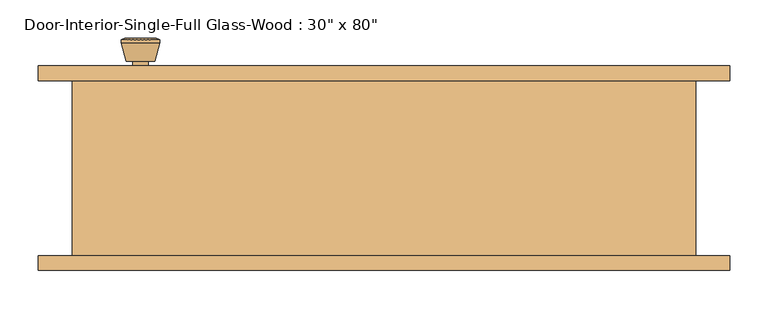
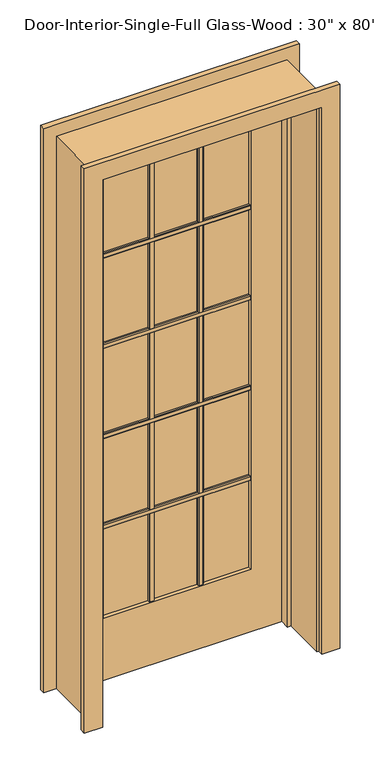
"""IFC4 building model written with IfcOpenShell, lengths in millimetres: door geometry."""

from ifc_helpers import new_model, si_unit, point, frame, frame_2d, origin, place, context, project, spatial, polyline, circle_curve, trimmed, segment, composite_curve, outline, extrude, faceted_brep, source, transform, mapped, element, save
from ifc_brep_helpers import plane_surface, cylinder_surface, revolved_surface, advanced_brep


def door_efd3daa1(model_context):
    return source(origin(), model_context, "Body", "SolidModel", [
        extrude(outline(polyline([(97.155, 1586.23), (103.505, 1586.23), (106.68, 1583.055), (106.68, 1570.355), (103.505, 1567.18), (97.155, 1567.18), (97.155, 1586.23)])), frame((-260.35, 0.0, 0.0), z_axis=(1.0, 0.0, 0.0), x_axis=(0.0, 1.0, 0.0)), (0.0, 0.0, 1.0), 520.7),
        extrude(outline(polyline([(97.155, 1249.9975), (103.505, 1249.9975), (106.68, 1246.8225), (106.68, 1234.1225), (103.505, 1230.9475), (97.155, 1230.9475), (97.155, 1249.9975)])), frame((-260.35, 0.0, 0.0), z_axis=(1.0, 0.0, 0.0), x_axis=(0.0, 1.0, 0.0)), (0.0, 0.0, 1.0), 520.7),
        extrude(outline(polyline([(97.155, 913.765), (103.505, 913.765), (106.68, 910.59), (106.68, 897.89), (103.505, 894.715), (97.155, 894.715), (97.155, 913.765)])), frame((-260.35, 0.0, 0.0), z_axis=(1.0, 0.0, 0.0), x_axis=(0.0, 1.0, 0.0)), (0.0, 0.0, 1.0), 520.7),
        extrude(outline(polyline([(97.155, 577.5325), (103.505, 577.5325), (106.68, 574.3575), (106.68, 561.6575), (103.505, 558.4825), (97.155, 558.4825), (97.155, 577.5325)])), frame((-260.35, 0.0, 0.0), z_axis=(1.0, 0.0, 0.0), x_axis=(0.0, 1.0, 0.0)), (0.0, 0.0, 1.0), 520.7),
        extrude(outline(polyline([(77.2583333, 97.155), (77.2583333, 103.505), (80.4333333, 106.68), (93.1333333, 106.68), (96.3083333, 103.505), (96.3083333, 97.155), (77.2583333, 97.155)])), frame((0.0, 0.0, 231.775), z_axis=(0.0, 0.0, 1.0), x_axis=(1.0, 0.0, 0.0)), (0.0, 0.0, 1.0), 1681.1625),
        extrude(outline(polyline([(-96.3083333, 97.155), (-96.3083333, 103.505), (-93.1333333, 106.68), (-80.4333333, 106.68), (-77.2583333, 103.505), (-77.2583333, 97.155), (-96.3083333, 97.155)])), frame((0.0, 0.0, 231.775), z_axis=(0.0, 0.0, 1.0), x_axis=(1.0, 0.0, 0.0)), (0.0, 0.0, 1.0), 1681.1625),
        extrude(outline(polyline([(90.17, 1586.23), (90.17, 1567.18), (83.82, 1567.18), (80.645, 1570.355), (80.645, 1583.055), (83.82, 1586.23), (90.17, 1586.23)])), frame((-260.35, 0.0, 0.0), z_axis=(1.0, 0.0, 0.0), x_axis=(0.0, 1.0, 0.0)), (0.0, 0.0, 1.0), 520.7),
        extrude(outline(polyline([(90.17, 1249.9975), (90.17, 1230.9475), (83.82, 1230.9475), (80.645, 1234.1225), (80.645, 1246.8225), (83.82, 1249.9975), (90.17, 1249.9975)])), frame((-260.35, 0.0, 0.0), z_axis=(1.0, 0.0, 0.0), x_axis=(0.0, 1.0, 0.0)), (0.0, 0.0, 1.0), 520.7),
        extrude(outline(polyline([(90.17, 913.765), (90.17, 894.715), (83.82, 894.715), (80.645, 897.89), (80.645, 910.59), (83.82, 913.765), (90.17, 913.765)])), frame((-260.35, 0.0, 0.0), z_axis=(1.0, 0.0, 0.0), x_axis=(0.0, 1.0, 0.0)), (0.0, 0.0, 1.0), 520.7),
        extrude(outline(polyline([(90.17, 577.5325), (90.17, 558.4825), (83.82, 558.4825), (80.645, 561.6575), (80.645, 574.3575), (83.82, 577.5325), (90.17, 577.5325)])), frame((-260.35, 0.0, 0.0), z_axis=(1.0, 0.0, 0.0), x_axis=(0.0, 1.0, 0.0)), (0.0, 0.0, 1.0), 520.7),
        extrude(outline(polyline([(77.2583333, 90.17), (96.3083333, 90.17), (96.3083333, 83.82), (93.1333333, 80.645), (80.4333333, 80.645), (77.2583333, 83.82), (77.2583333, 90.17)])), frame((0.0, 0.0, 231.775), z_axis=(0.0, 0.0, 1.0), x_axis=(1.0, 0.0, 0.0)), (0.0, 0.0, 1.0), 1681.1625),
        extrude(outline(polyline([(-96.3083333, 90.17), (-77.2583333, 90.17), (-77.2583333, 83.82), (-80.4333333, 80.645), (-93.1333333, 80.645), (-96.3083333, 83.82), (-96.3083333, 90.17)])), frame((0.0, 0.0, 231.775), z_axis=(0.0, 0.0, 1.0), x_axis=(1.0, 0.0, 0.0)), (0.0, 0.0, 1.0), 1681.1625),
        advanced_brep(
        [(-317.5, 70.2, 914.4), (-307.5, 70.2, 914.4), (-327.5, 70.2, 914.4), (-297.0241324, 21.2, 914.4), (-317.5, 21.2, 914.4), (-337.9758676, 21.2, 914.4), (-292.5, 23.0278681, 914.4), (-342.5, 23.0278681, 914.4), (-292.5, 26.4915463, 914.4), (-342.5, 26.4915463, 914.4), (-298.863764, 51.2, 914.4), (-336.136236, 51.2, 914.4), (-307.5, 51.2, 914.4), (-327.5, 51.2, 914.4)],
        [
            (0, 1),
            (1, 2, circle_curve(frame((-317.5, 70.2, 914.4), z_axis=(0.0, 1.0, 0.0), x_axis=(-1.0, 0.0, 0.0)), 10.0)),
            (2, 0),
            (2, 1, circle_curve(frame((-317.5, 70.2, 914.4), z_axis=(0.0, 1.0, 0.0), x_axis=(-1.0, 0.0, 0.0)), 10.0)),
            (3, 4),
            (4, 5),
            (5, 3, circle_curve(frame((-317.5, 21.2, 914.4), z_axis=(0.0, -1.0, 0.0), x_axis=(-1.0, 0.0, 0.0)), 20.4758676)),
            (3, 5, circle_curve(frame((-317.5, 21.2, 914.4), z_axis=(0.0, -1.0, 0.0), x_axis=(-1.0, 0.0, 0.0)), 20.4758676)),
            (6, 3),
            (5, 7),
            (7, 6, circle_curve(frame((-317.5, 23.0278681, 914.4), z_axis=(0.0, -1.0, 0.0), x_axis=(-1.0, 0.0, 0.0)), 25.0)),
            (6, 7, circle_curve(frame((-317.5, 23.0278681, 914.4), z_axis=(0.0, -1.0, 0.0), x_axis=(-1.0, 0.0, 0.0)), 25.0)),
            (8, 6),
            (7, 9),
            (9, 8, circle_curve(frame((-317.5, 26.4915463, 914.4), z_axis=(0.0, -1.0, 0.0), x_axis=(-1.0, 0.0, 0.0)), 25.0)),
            (8, 9, circle_curve(frame((-317.5, 26.4915463, 914.4), z_axis=(0.0, -1.0, 0.0), x_axis=(-1.0, 0.0, 0.0)), 25.0)),
            (10, 8),
            (9, 11),
            (11, 10, circle_curve(frame((-317.5, 51.2, 914.4), z_axis=(0.0, -1.0, 0.0), x_axis=(-1.0, 0.0, 0.0)), 18.636236)),
            (10, 11, circle_curve(frame((-317.5, 51.2, 914.4), z_axis=(0.0, -1.0, 0.0), x_axis=(-1.0, 0.0, 0.0)), 18.636236)),
            (12, 10),
            (11, 13),
            (13, 12, circle_curve(frame((-317.5, 51.2, 914.4), z_axis=(0.0, -1.0, 0.0), x_axis=(-1.0, 0.0, 0.0)), 10.0)),
            (12, 13, circle_curve(frame((-317.5, 51.2, 914.4), z_axis=(0.0, -1.0, 0.0), x_axis=(-1.0, 0.0, 0.0)), 10.0)),
            (1, 12),
            (13, 2),
        ],
        [
            plane_surface(frame((-317.5, 70.2, 914.4), z_axis=(0.0, 1.0, 0.0), x_axis=(-1.0, 0.0, 0.0))),
            plane_surface(frame((-317.5, 21.2, 914.4), z_axis=(0.0, -1.0, 0.0), x_axis=(-1.0, 0.0, 0.0))),
            revolved_surface(polyline([(-337.9758676, 21.2, 914.4), (-342.5, 23.0278681, 914.4)]), (-317.5, 70.2, 914.4), (0.0, 1.0, 0.0)),
            cylinder_surface(frame((-317.5, 70.2, 914.4), z_axis=(0.0, 1.0, 0.0), x_axis=(-1.0, 0.0, 0.0)), 25.0),
            revolved_surface(polyline([(-342.5, 26.4915463, 914.4), (-336.136236, 51.2, 914.4)]), (-317.5, 70.2, 914.4), (0.0, 1.0, 0.0)),
            plane_surface(frame((-317.5, 51.2, 914.4), z_axis=(0.0, 1.0, 0.0), x_axis=(-1.0, 0.0, 0.0))),
            cylinder_surface(frame((-317.5, 70.2, 914.4), z_axis=(0.0, 1.0, 0.0), x_axis=(-1.0, 0.0, 0.0)), 10.0),
        ],
        [
            (0, [[1, 2, 3]]),
            (0, [[-3, 4, -1]]),
            (1, [[5, 6, 7]]),
            (1, [[-6, -5, 8]]),
            (2, [[9, -7, 10, 11]]),
            (2, [[-10, -8, -9, 12]]),
            (3, [[13, -11, 14, 15]]),
            (3, [[-14, -12, -13, 16]]),
            (4, [[17, -15, 18, 19]]),
            (4, [[-18, -16, -17, 20]]),
            (5, [[21, -19, 22, 23]]),
            (5, [[-22, -20, -21, 24]]),
            (6, [[25, -23, 26, -2]]),
            (6, [[-26, -24, -25, -4]]),
        ],
    ),
        extrude(outline(composite_curve([segment(trimmed(circle_curve(frame_2d((914.4, -317.5)), 30.0), [point((914.4, -347.5))], [point((914.4, -287.5))], False, "CARTESIAN"), True, "CONTINUOUS"), segment(trimmed(circle_curve(frame_2d((914.4, -317.5)), 30.0), [point((914.4, -287.5))], [point((914.4, -347.5))], False, "CARTESIAN"), True, "CONTINUOUS")], self_intersect=False)), frame((0.0, 70.2, 0.0), z_axis=(0.0, 1.0, 0.0), x_axis=(0.0, 0.0, 1.0)), (0.0, 0.0, 1.0), 6.0),
        advanced_brep(
        [(-317.5, 117.125, 914.4), (-327.5, 117.125, 914.4), (-307.5, 117.125, 914.4), (-297.0241324, 166.125, 914.4), (-337.9758676, 166.125, 914.4), (-317.5, 166.125, 914.4), (-292.5, 164.2971319, 914.4), (-342.5, 164.2971319, 914.4), (-292.5, 160.8334537, 914.4), (-342.5, 160.8334537, 914.4), (-298.863764, 136.125, 914.4), (-336.136236, 136.125, 914.4), (-307.5, 136.125, 914.4), (-327.5, 136.125, 914.4)],
        [
            (0, 1),
            (1, 2, circle_curve(frame((-317.5, 117.125, 914.4), z_axis=(0.0, -1.0, 0.0), x_axis=(-1.0, 0.0, 0.0)), 10.0)),
            (2, 0),
            (2, 1, circle_curve(frame((-317.5, 117.125, 914.4), z_axis=(0.0, -1.0, 0.0), x_axis=(-1.0, 0.0, 0.0)), 10.0)),
            (3, 4, circle_curve(frame((-317.5, 166.125, 914.4), z_axis=(0.0, 1.0, 0.0), x_axis=(-1.0, 0.0, 0.0)), 20.4758676)),
            (4, 5),
            (5, 3),
            (4, 3, circle_curve(frame((-317.5, 166.125, 914.4), z_axis=(0.0, 1.0, 0.0), x_axis=(-1.0, 0.0, 0.0)), 20.4758676)),
            (6, 7, circle_curve(frame((-317.5, 164.2971319, 914.4), z_axis=(0.0, 1.0, 0.0), x_axis=(-1.0, 0.0, 0.0)), 25.0)),
            (7, 4),
            (3, 6),
            (7, 6, circle_curve(frame((-317.5, 164.2971319, 914.4), z_axis=(0.0, 1.0, 0.0), x_axis=(-1.0, 0.0, 0.0)), 25.0)),
            (8, 9, circle_curve(frame((-317.5, 160.8334537, 914.4), z_axis=(0.0, 1.0, 0.0), x_axis=(-1.0, 0.0, 0.0)), 25.0)),
            (9, 7),
            (6, 8),
            (9, 8, circle_curve(frame((-317.5, 160.8334537, 914.4), z_axis=(0.0, 1.0, 0.0), x_axis=(-1.0, 0.0, 0.0)), 25.0)),
            (10, 11, circle_curve(frame((-317.5, 136.125, 914.4), z_axis=(0.0, 1.0, 0.0), x_axis=(-1.0, 0.0, 0.0)), 18.636236)),
            (11, 9),
            (8, 10),
            (11, 10, circle_curve(frame((-317.5, 136.125, 914.4), z_axis=(0.0, 1.0, 0.0), x_axis=(-1.0, 0.0, 0.0)), 18.636236)),
            (12, 13, circle_curve(frame((-317.5, 136.125, 914.4), z_axis=(0.0, 1.0, 0.0), x_axis=(-1.0, 0.0, 0.0)), 10.0)),
            (13, 11),
            (10, 12),
            (13, 12, circle_curve(frame((-317.5, 136.125, 914.4), z_axis=(0.0, 1.0, 0.0), x_axis=(-1.0, 0.0, 0.0)), 10.0)),
            (1, 13),
            (12, 2),
        ],
        [
            plane_surface(frame((-317.5, 117.125, 914.4), z_axis=(0.0, -1.0, 0.0), x_axis=(-1.0, 0.0, 0.0))),
            plane_surface(frame((-317.5, 166.125, 914.4), z_axis=(0.0, 1.0, 0.0), x_axis=(-1.0, 0.0, 0.0))),
            revolved_surface(polyline([(-337.9758676, 166.125, 914.4), (-342.5, 164.2971319, 914.4)]), (-317.5, 117.125, 914.4), (0.0, -1.0, 0.0)),
            cylinder_surface(frame((-317.5, 117.125, 914.4), z_axis=(0.0, -1.0, 0.0), x_axis=(-1.0, 0.0, 0.0)), 25.0),
            revolved_surface(polyline([(-342.5, 160.8334537, 914.4), (-336.136236, 136.125, 914.4)]), (-317.5, 117.125, 914.4), (0.0, -1.0, 0.0)),
            plane_surface(frame((-317.5, 136.125, 914.4), z_axis=(0.0, -1.0, 0.0), x_axis=(-1.0, 0.0, 0.0))),
            cylinder_surface(frame((-317.5, 117.125, 914.4), z_axis=(0.0, -1.0, 0.0), x_axis=(-1.0, 0.0, 0.0)), 10.0),
        ],
        [
            (0, [[1, 2, 3]]),
            (0, [[-3, 4, -1]]),
            (1, [[5, 6, 7]]),
            (1, [[8, -7, -6]]),
            (2, [[9, 10, -5, 11]]),
            (2, [[12, -11, -8, -10]]),
            (3, [[13, 14, -9, 15]]),
            (3, [[16, -15, -12, -14]]),
            (4, [[17, 18, -13, 19]]),
            (4, [[20, -19, -16, -18]]),
            (5, [[21, 22, -17, 23]]),
            (5, [[24, -23, -20, -22]]),
            (6, [[-2, 25, -21, 26]]),
            (6, [[-4, -26, -24, -25]]),
        ],
    ),
        extrude(outline(composite_curve([segment(trimmed(circle_curve(frame_2d((914.4, -317.5)), 30.0), [point((914.4, -347.5))], [point((914.4, -287.5))], False, "CARTESIAN"), True, "CONTINUOUS"), segment(trimmed(circle_curve(frame_2d((914.4, -317.5)), 30.0), [point((914.4, -287.5))], [point((914.4, -347.5))], False, "CARTESIAN"), True, "CONTINUOUS")], self_intersect=False)), frame((0.0, 111.125, 0.0), z_axis=(0.0, 1.0, 0.0), x_axis=(0.0, 0.0, 1.0)), (0.0, 0.0, 1.0), 6.0),
        extrude(outline(polyline([(2032.0, -381.0), (0.0, -381.0), (0.0, 381.0), (2032.0, 381.0), (2032.0, -381.0)]), holes=[polyline([(1912.9375, -260.35), (1912.9375, 260.35), (231.775, 260.35), (231.775, -260.35), (1912.9375, -260.35)])]), frame((0.0, 76.2, 0.0), z_axis=(0.0, 1.0, 0.0), x_axis=(0.0, 0.0, 1.0)), (0.0, 0.0, 1.0), 34.925),
        faceted_brep([(406.4, 111.125, 0.0), (406.4, -117.475, 0.0), (381.0, -117.475, 0.0), (381.0, 41.275, 0.0), (368.3, 41.275, 0.0), (368.3, 76.2, 0.0), (381.0, 76.2, 0.0), (381.0, 111.125, 0.0), (406.4, 111.125, 2057.4), (406.4, -117.475, 2057.4), (-406.4, -117.475, 2057.4), (-406.4, -117.475, 0.0), (-381.0, -117.475, 0.0), (-381.0, -117.475, 2032.0), (381.0, -117.475, 2032.0), (381.0, 41.275, 2032.0), (-381.0, 41.275, 2032.0), (-381.0, 41.275, 0.0), (-368.3, 41.275, 0.0), (-368.3, 41.275, 2019.3), (368.3, 41.275, 2019.3), (368.3, 76.2, 2019.3), (-368.3, 76.2, 2019.3), (-368.3, 76.2, 0.0), (-381.0, 76.2, 0.0), (-381.0, 76.2, 2032.0), (381.0, 76.2, 2032.0), (381.0, 111.125, 2032.0), (-381.0, 111.125, 2032.0), (-381.0, 111.125, 0.0), (-406.4, 111.125, 0.0), (-406.4, 111.125, 2057.4)], [[[0, 1, 2, 3, 4, 5, 6, 7]], [[1, 0, 8, 9]], [[2, 1, 9, 10, 11, 12, 13, 14]], [[3, 2, 14, 15]], [[4, 3, 15, 16, 17, 18, 19, 20]], [[5, 4, 20, 21]], [[6, 5, 21, 22, 23, 24, 25, 26]], [[7, 6, 26, 27]], [[0, 7, 27, 28, 29, 30, 31, 8]], [[9, 8, 31, 10]], [[15, 14, 13, 16]], [[21, 20, 19, 22]], [[27, 26, 25, 28]], [[30, 29, 24, 23, 18, 17, 12, 11]], [[10, 31, 30, 11]], [[16, 13, 12, 17]], [[22, 19, 18, 23]], [[28, 25, 24, 29]]]),
        extrude(outline(polyline([(260.35, 90.17), (-260.35, 90.17), (-260.35, 97.155), (260.35, 97.155), (260.35, 90.17)])), frame((0.0, 0.0, 231.775), z_axis=(0.0, 0.0, 1.0), x_axis=(1.0, 0.0, 0.0)), (0.0, 0.0, 1.0), 1681.1625),
        extrude(outline(polyline([(0.0, 387.35), (0.0, 450.85), (2101.85, 450.85), (2101.85, -450.85), (0.0, -450.85), (0.0, -387.35), (2038.35, -387.35), (2038.35, 387.35), (0.0, 387.35)])), frame((0.0, -136.525, 0.0), z_axis=(0.0, 1.0, 0.0), x_axis=(0.0, 0.0, 1.0)), (0.0, 0.0, 1.0), 19.05),
        extrude(outline(polyline([(0.0, 387.35), (0.0, 450.85), (2101.85, 450.85), (2101.85, -450.85), (0.0, -450.85), (0.0, -387.35), (2038.35, -387.35), (2038.35, 387.35), (0.0, 387.35)])), frame((0.0, 111.125, 0.0), z_axis=(0.0, 1.0, 0.0), x_axis=(0.0, 0.0, 1.0)), (0.0, 0.0, 1.0), 19.05),
    ])


if __name__ == "__main__":
    model = new_model("IFC4")
    model_context = context("Model", 3, world=origin())
    ifc_project = project(units=[si_unit("LENGTHUNIT", "METRE", prefix="MILLI")], contexts=[model_context])
    site = spatial("IfcSite", under=ifc_project)
    building = spatial("IfcBuilding", under=site)
    placement = place(None, origin())
    door_shape = door_efd3daa1(model_context)
    element("IfcDoor", 1, ObjectType="Door-Interior-Single-Full Glass-Wood : 30\" x 80\"", at=placement, inside=building, context=model_context, shape_type="MappedRepresentation", body=[
        mapped(door_shape, transform((0.0, 0.0, 0.0), x_axis=(1.0, 0.0, 0.0), y_axis=(0.0, 1.0, 0.0), z_axis=(0.0, 0.0, 1.0))),
    ])
    save(model, "model.ifc")

# Revit data of these elements
# Type "Door-Interior-Single-Full Glass-Wood : 30\" x 80\""
#   Type Mark = "10"
#   Assembly Code = "C1020300"
#   Analytic Construction = "Wood frame with single clear glass"
#   Top Rail = 0' - 4 11/16"
#   Thickness = 0' - 1 3/8"
#   Thermal Resistance (R) = 1.0102 (h·ft²·°F)/BTU
#   Swing Angle [instance default] = 90.00°
#   Stiles = 0' - 4 3/4"
#   Rough Width = 2' - 8"
#   Rough Height = 6' - 9"
#   Height = 6' - 8"
#   Width = 2' - 6"
#   Heat Transfer Coefficient (U) = 0.9900 BTU/(h·ft²·°F)
#   Bottom Rail = 0' - 9 1/8"
#   Show Grill [instance default] = yes
#   Trim Material = Cherry
#   Panel Material = Cherry
#   Frame Material = Cherry
#   Door Handle Material = Aluminum
#   Visual Light Transmittance = 0
#   Solar Heat Gain Coefficient = 0
#   Wall Closure = (empty or 0)
#   Function = (empty or 0)
# Element 1 (IfcDoor, "Door-Interior-Single-Full Glass-Wood : 30\" x 80\"")
#   Materials on its faces: "Cherry", "Aluminum", "Glass"
# Materials
#   "Cherry": class "Wood", colour RGB 226 177 128, transparency 0, Description = "Prunus Serotina", Cost = 0
#   "Aluminum": class "Metal", colour RGB 247 247 247, transparency 0, Description = "Aluminum 6061", Cost = 0
#   "Glass": class "Glass", colour RGB 0 128 192, transparency 0.75, Description = "Soda Lime Glass", Cost = 0
